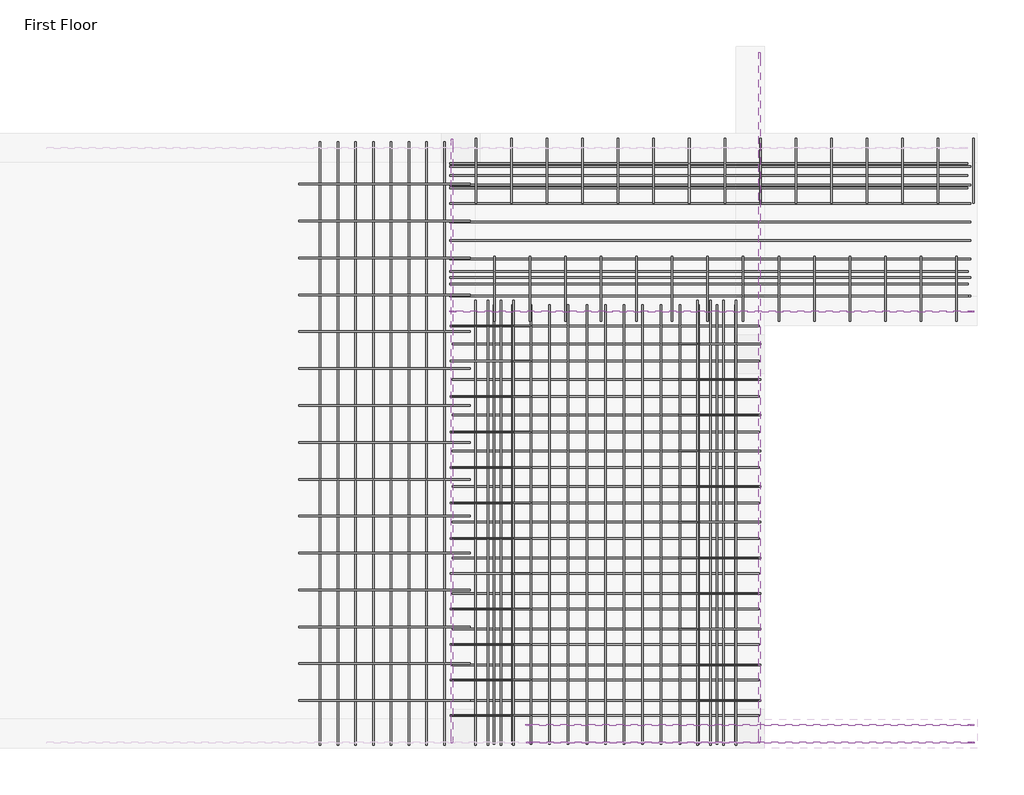
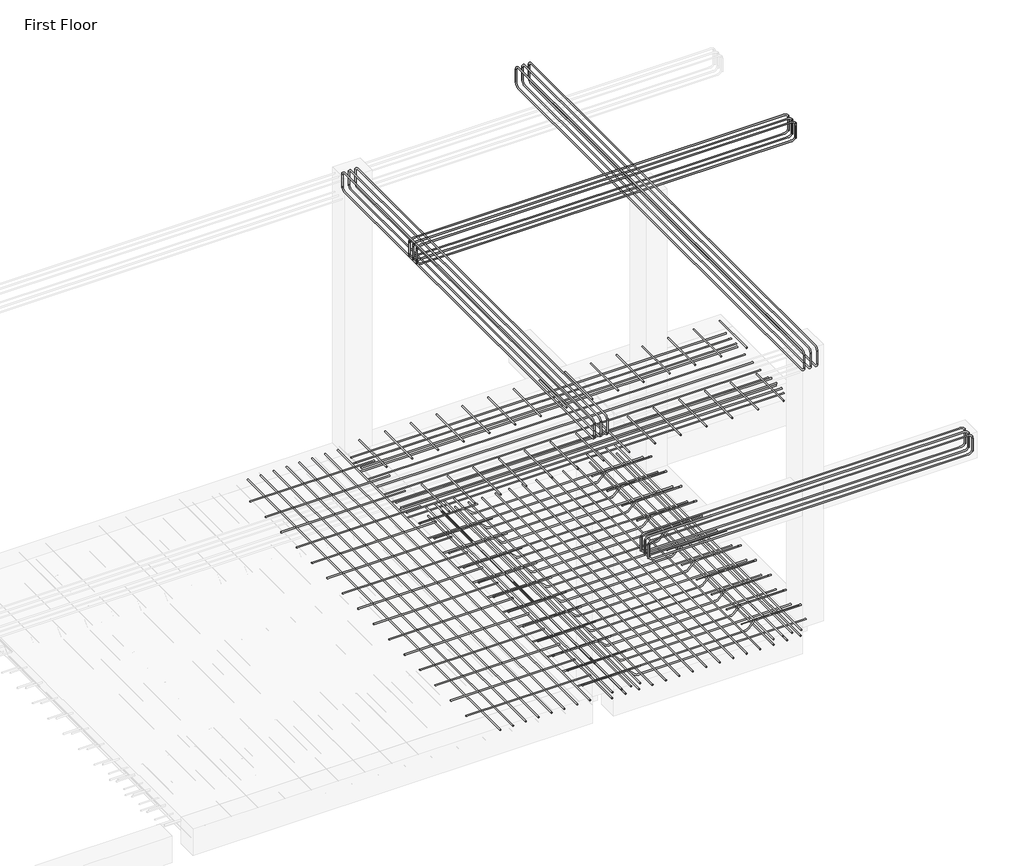
# One storey, part 4 of 4: 22 reinforcing bars.
"""IFC4 building model written with IfcOpenShell, lengths in millimetres."""

from ifc_helpers import new_model, si_unit, point, frame, origin, place, context, project, spatial, polyline, circle_curve, trimmed, segment, composite_curve, source, transform, mapped, element, save
from ifc_brep_helpers import swept_disk

model = new_model("IFC4")

# Units and contexts
model_context = context("Model", 3, world=origin())
ifc_project = project(units=[si_unit("LENGTHUNIT", "METRE", prefix="MILLI")], contexts=[model_context])

# Site, building, storey
site = spatial("IfcSite", under=ifc_project)
building = spatial("IfcBuilding", under=site)
storey = spatial("IfcBuildingStorey", under=building, Name="First Floor", Elevation=3200.4)

# Reinforcing bars
placement = place(None, origin())
reinforcing_bar_shape = source(origin(), model_context, "Body", "SolidModel", [
    swept_disk(composite_curve([segment(polyline([(1700.4887526, 5017.2334631, 6163.6994949), (1700.4887526, 5017.2334631, 6311.6994949)]), True, "CONTINUOUS"), segment(trimmed(circle_curve(frame((1700.4887526, 4971.2334631, 6311.6994949), z_axis=(1.0, 0.0, 0.0), x_axis=(0.0, 46.0, 0.0)), 46.0), [point((1700.4887526, 5017.2334631, 6311.6994949))], [point((1700.4887526, 4971.2334631, 6357.6994949))], True, "CARTESIAN"), True, "CONTINUOUS"), segment(polyline([(1700.4887526, 4971.2334631, 6357.6994949), (1700.4887526, 278.4334631, 6357.6994949)]), True, "CONTINUOUS"), segment(trimmed(circle_curve(frame((1700.4887526, 278.4334631, 6311.6994949), z_axis=(1.0, 0.0, 0.0), x_axis=(0.0, 0.0, 46.0)), 46.0), [point((1700.4887526, 278.4334631, 6357.6994949))], [point((1700.4887526, 232.4334631, 6311.6994949))], True, "CARTESIAN"), True, "CONTINUOUS"), segment(polyline([(1700.4887526, 232.4334631, 6311.6994949), (1700.4887526, 232.4334631, 6163.6994949)]), True, "CONTINUOUS")], self_intersect=False), 6.0),
])
element("IfcReinforcingBar", 1, at=placement, inside=storey, context=model_context, shape_type="MappedRepresentation", body=[
    mapped(reinforcing_bar_shape, transform((0.0, 0.0, 0.0), x_axis=(1.0, 0.0, 0.0), y_axis=(0.0, 1.0, 0.0), z_axis=(0.0, 0.0, 1.0))),
    mapped(reinforcing_bar_shape, transform((71.1994949, 0.0, 0.0), x_axis=(1.0, 0.0, 0.0), y_axis=(0.0, 1.0, 0.0), z_axis=(0.0, 0.0, 1.0))),
    mapped(reinforcing_bar_shape, transform((142.3989899, 0.0, 0.0), x_axis=(1.0, 0.0, 0.0), y_axis=(0.0, 1.0, 0.0), z_axis=(0.0, 0.0, 1.0))),
])
reinforcing_bar_2_shape = source(origin(), model_context, "Body", "SolidModel", [
    swept_disk(composite_curve([segment(polyline([(1700.4887526, 5017.2334631, 6333.1005051), (1700.4887526, 5017.2334631, 6185.1005051)]), True, "CONTINUOUS"), segment(trimmed(circle_curve(frame((1700.4887526, 4971.2334631, 6185.1005051), z_axis=(-1.0, 0.0, 0.0), x_axis=(0.0, 46.0, 0.0)), 46.0), [point((1700.4887526, 5017.2334631, 6185.1005051))], [point((1700.4887526, 4971.2334631, 6139.1005051))], True, "CARTESIAN"), True, "CONTINUOUS"), segment(polyline([(1700.4887526, 4971.2334631, 6139.1005051), (1700.4887526, 278.4334631, 6139.1005051)]), True, "CONTINUOUS"), segment(trimmed(circle_curve(frame((1700.4887526, 278.4334631, 6185.1005051), z_axis=(-1.0, 0.0, 0.0), x_axis=(0.0, 0.0, -46.0)), 46.0), [point((1700.4887526, 278.4334631, 6139.1005051))], [point((1700.4887526, 232.4334631, 6185.1005051))], True, "CARTESIAN"), True, "CONTINUOUS"), segment(polyline([(1700.4887526, 232.4334631, 6185.1005051), (1700.4887526, 232.4334631, 6333.1005051)]), True, "CONTINUOUS")], self_intersect=False), 6.0),
])
element("IfcReinforcingBar", 2, at=placement, inside=storey, context=model_context, shape_type="MappedRepresentation", body=[
    mapped(reinforcing_bar_2_shape, transform((0.0, 0.0, 0.0), x_axis=(1.0, 0.0, 0.0), y_axis=(0.0, 1.0, 0.0), z_axis=(0.0, 0.0, 1.0))),
    mapped(reinforcing_bar_2_shape, transform((71.1994949, 0.0, 0.0), x_axis=(1.0, 0.0, 0.0), y_axis=(0.0, 1.0, 0.0), z_axis=(0.0, 0.0, 1.0))),
    mapped(reinforcing_bar_2_shape, transform((142.3989899, 0.0, 0.0), x_axis=(1.0, 0.0, 0.0), y_axis=(0.0, 1.0, 0.0), z_axis=(0.0, 0.0, 1.0))),
])
reinforcing_bar_3_shape = source(origin(), model_context, "Body", "SolidModel", [
    swept_disk(composite_curve([segment(polyline([(3999.1887526, 5705.3580501, 6163.6994949), (3999.1887526, 5705.3580501, 6311.6994949)]), True, "CONTINUOUS"), segment(trimmed(circle_curve(frame((3999.1887526, 5659.3580501, 6311.6994949), z_axis=(1.0, 0.0, 0.0), x_axis=(0.0, 46.0, 0.0)), 46.0), [point((3999.1887526, 5705.3580501, 6311.6994949))], [point((3999.1887526, 5659.3580501, 6357.6994949))], True, "CARTESIAN"), True, "CONTINUOUS"), segment(polyline([(3999.1887526, 5659.3580501, 6357.6994949), (3999.1887526, 278.4334631, 6357.6994949)]), True, "CONTINUOUS"), segment(trimmed(circle_curve(frame((3999.1887526, 278.4334631, 6311.6994949), z_axis=(1.0, 0.0, 0.0), x_axis=(0.0, 0.0, 46.0)), 46.0), [point((3999.1887526, 278.4334631, 6357.6994949))], [point((3999.1887526, 232.4334631, 6311.6994949))], True, "CARTESIAN"), True, "CONTINUOUS"), segment(polyline([(3999.1887526, 232.4334631, 6311.6994949), (3999.1887526, 232.4334631, 6163.6994949)]), True, "CONTINUOUS")], self_intersect=False), 6.0),
])
element("IfcReinforcingBar", 3, at=placement, inside=storey, context=model_context, shape_type="MappedRepresentation", body=[
    mapped(reinforcing_bar_3_shape, transform((0.0, 0.0, 0.0), x_axis=(1.0, 0.0, 0.0), y_axis=(0.0, 1.0, 0.0), z_axis=(0.0, 0.0, 1.0))),
    mapped(reinforcing_bar_3_shape, transform((71.1994949, 0.0, 0.0), x_axis=(1.0, 0.0, 0.0), y_axis=(0.0, 1.0, 0.0), z_axis=(0.0, 0.0, 1.0))),
    mapped(reinforcing_bar_3_shape, transform((142.3989899, 0.0, 0.0), x_axis=(1.0, 0.0, 0.0), y_axis=(0.0, 1.0, 0.0), z_axis=(0.0, 0.0, 1.0))),
])
reinforcing_bar_4_shape = source(origin(), model_context, "Body", "SolidModel", [
    swept_disk(composite_curve([segment(polyline([(3999.1887526, 5703.3830416, 6318.1005051), (3999.1887526, 5703.3830416, 6170.1005051)]), True, "CONTINUOUS"), segment(trimmed(circle_curve(frame((3999.1887526, 5657.3830416, 6170.1005051), z_axis=(-1.0, 0.0, 0.0), x_axis=(0.0, 46.0, 0.0)), 46.0), [point((3999.1887526, 5703.3830416, 6170.1005051))], [point((3999.1887526, 5657.3830416, 6124.1005051))], True, "CARTESIAN"), True, "CONTINUOUS"), segment(polyline([(3999.1887526, 5657.3830416, 6124.1005051), (3999.1887526, 278.4334631, 6124.1005051)]), True, "CONTINUOUS"), segment(trimmed(circle_curve(frame((3999.1887526, 278.4334631, 6170.1005051), z_axis=(-1.0, 0.0, 0.0), x_axis=(0.0, 0.0, -46.0)), 46.0), [point((3999.1887526, 278.4334631, 6124.1005051))], [point((3999.1887526, 232.4334631, 6170.1005051))], True, "CARTESIAN"), True, "CONTINUOUS"), segment(polyline([(3999.1887526, 232.4334631, 6170.1005051), (3999.1887526, 232.4334631, 6318.1005051)]), True, "CONTINUOUS")], self_intersect=False), 6.0),
])
element("IfcReinforcingBar", 4, at=placement, inside=storey, context=model_context, shape_type="MappedRepresentation", body=[
    mapped(reinforcing_bar_4_shape, transform((0.0, 0.0, 0.0), x_axis=(1.0, 0.0, 0.0), y_axis=(0.0, 1.0, 0.0), z_axis=(0.0, 0.0, 1.0))),
    mapped(reinforcing_bar_4_shape, transform((71.1994949, 0.0, 0.0), x_axis=(1.0, 0.0, 0.0), y_axis=(0.0, 1.0, 0.0), z_axis=(0.0, 0.0, 1.0))),
    mapped(reinforcing_bar_4_shape, transform((142.3989899, 0.0, 0.0), x_axis=(1.0, 0.0, 0.0), y_axis=(0.0, 1.0, 0.0), z_axis=(0.0, 0.0, 1.0))),
])
reinforcing_bar_5_shape = source(origin(), model_context, "Body", "SolidModel", [
    swept_disk(composite_curve([segment(polyline([(5841.2691711, 3584.0814555, 6161.9520076), (5841.2691711, 3584.0814555, 6309.9520076)]), True, "CONTINUOUS"), segment(trimmed(circle_curve(frame((5795.2691711, 3584.0814555, 6309.9520076), z_axis=(0.0, -1.0, 0.0), x_axis=(46.0, 0.0, 0.0)), 46.0), [point((5841.2691711, 3584.0814555, 6309.9520076))], [point((5795.2691711, 3584.0814555, 6355.9520076))], True, "CARTESIAN"), True, "CONTINUOUS"), segment(polyline([(5795.2691711, 3584.0814555, 6355.9520076), (1734.3882476, 3584.0814555, 6355.9520076)]), True, "CONTINUOUS"), segment(trimmed(circle_curve(frame((1734.3882476, 3584.0814555, 6309.9520076), z_axis=(0.0, -1.0, 0.0), x_axis=(0.0, 0.0, 46.0)), 46.0), [point((1734.3882476, 3584.0814555, 6355.9520076))], [point((1688.3882476, 3584.0814555, 6309.9520076))], True, "CARTESIAN"), True, "CONTINUOUS"), segment(polyline([(1688.3882476, 3584.0814555, 6309.9520076), (1688.3882476, 3584.0814555, 6161.9520076)]), True, "CONTINUOUS")], self_intersect=False), 6.0),
])
element("IfcReinforcingBar", 5, at=placement, inside=storey, context=model_context, shape_type="MappedRepresentation", body=[
    mapped(reinforcing_bar_5_shape, transform((0.0, 0.0, 0.0), x_axis=(1.0, 0.0, 0.0), y_axis=(0.0, 1.0, 0.0), z_axis=(0.0, 0.0, 1.0))),
    mapped(reinforcing_bar_5_shape, transform((0.0, 69.4520076, 0.0), x_axis=(1.0, 0.0, 0.0), y_axis=(0.0, 1.0, 0.0), z_axis=(0.0, 0.0, 1.0))),
    mapped(reinforcing_bar_5_shape, transform((0.0, 138.9040151, 0.0), x_axis=(1.0, 0.0, 0.0), y_axis=(0.0, 1.0, 0.0), z_axis=(0.0, 0.0, 1.0))),
])
reinforcing_bar_6_shape = source(origin(), model_context, "Body", "SolidModel", [
    swept_disk(composite_curve([segment(polyline([(5840.2625116, 3584.0814555, 6334.8479924), (5840.2625116, 3584.0814555, 6186.8479924)]), True, "CONTINUOUS"), segment(trimmed(circle_curve(frame((5794.2625116, 3584.0814555, 6186.8479924), z_axis=(0.0, 1.0, 0.0), x_axis=(46.0, 0.0, 0.0)), 46.0), [point((5840.2625116, 3584.0814555, 6186.8479924))], [point((5794.2625116, 3584.0814555, 6140.8479924))], True, "CARTESIAN"), True, "CONTINUOUS"), segment(polyline([(5794.2625116, 3584.0814555, 6140.8479924), (1734.3882476, 3584.0814555, 6140.8479924)]), True, "CONTINUOUS"), segment(trimmed(circle_curve(frame((1734.3882476, 3584.0814555, 6186.8479924), z_axis=(0.0, 1.0, 0.0), x_axis=(0.0, 0.0, -46.0)), 46.0), [point((1734.3882476, 3584.0814555, 6140.8479924))], [point((1688.3882476, 3584.0814555, 6186.8479924))], True, "CARTESIAN"), True, "CONTINUOUS"), segment(polyline([(1688.3882476, 3584.0814555, 6186.8479924), (1688.3882476, 3584.0814555, 6334.8479924)]), True, "CONTINUOUS")], self_intersect=False), 6.0),
])
element("IfcReinforcingBar", 6, at=placement, inside=storey, context=model_context, shape_type="MappedRepresentation", body=[
    mapped(reinforcing_bar_6_shape, transform((0.0, 0.0, 0.0), x_axis=(1.0, 0.0, 0.0), y_axis=(0.0, 1.0, 0.0), z_axis=(0.0, 0.0, 1.0))),
    mapped(reinforcing_bar_6_shape, transform((0.0, 69.4520076, 0.0), x_axis=(1.0, 0.0, 0.0), y_axis=(0.0, 1.0, 0.0), z_axis=(0.0, 0.0, 1.0))),
    mapped(reinforcing_bar_6_shape, transform((0.0, 138.9040151, 0.0), x_axis=(1.0, 0.0, 0.0), y_axis=(0.0, 1.0, 0.0), z_axis=(0.0, 0.0, 1.0))),
])
reinforcing_bar_7_shape = source(origin(), model_context, "Body", "SolidModel", [
    swept_disk(composite_curve([segment(polyline([(5841.2691711, 229.5339681, 4563.4994949), (5841.2691711, 229.5339681, 4711.4994949)]), True, "CONTINUOUS"), segment(trimmed(circle_curve(frame((5795.2691711, 229.5339681, 4711.4994949), z_axis=(0.0, -1.0, 0.0), x_axis=(46.0, 0.0, 0.0)), 46.0), [point((5841.2691711, 229.5339681, 4711.4994949))], [point((5795.2691711, 229.5339681, 4757.4994949))], True, "CARTESIAN"), True, "CONTINUOUS"), segment(polyline([(5795.2691711, 229.5339681, 4757.4994949), (2337.5636354, 229.5339681, 4757.4994949)]), True, "CONTINUOUS"), segment(trimmed(circle_curve(frame((2337.5636354, 229.5339681, 4711.4994949), z_axis=(0.0, -1.0, 0.0), x_axis=(0.0, 0.0, 46.0)), 46.0), [point((2337.5636354, 229.5339681, 4757.4994949))], [point((2291.5636354, 229.5339681, 4711.4994949))], True, "CARTESIAN"), True, "CONTINUOUS"), segment(polyline([(2291.5636354, 229.5339681, 4711.4994949), (2291.5636354, 229.5339681, 4563.4994949)]), True, "CONTINUOUS")], self_intersect=False), 6.0),
])
element("IfcReinforcingBar", 7, at=placement, inside=storey, context=model_context, shape_type="MappedRepresentation", body=[
    mapped(reinforcing_bar_7_shape, transform((0.0, 0.0, 0.0), x_axis=(1.0, 0.0, 0.0), y_axis=(0.0, 1.0, 0.0), z_axis=(0.0, 0.0, 1.0))),
    mapped(reinforcing_bar_7_shape, transform((0.0, 71.1994949, 0.0), x_axis=(1.0, 0.0, 0.0), y_axis=(0.0, 1.0, 0.0), z_axis=(0.0, 0.0, 1.0))),
    mapped(reinforcing_bar_7_shape, transform((0.0, 142.3989899, 0.0), x_axis=(1.0, 0.0, 0.0), y_axis=(0.0, 1.0, 0.0), z_axis=(0.0, 0.0, 1.0))),
])
reinforcing_bar_8_shape = source(origin(), model_context, "Body", "SolidModel", [
    swept_disk(composite_curve([segment(polyline([(5840.2625116, 229.5339681, 4732.9005051), (5840.2625116, 229.5339681, 4584.9005051)]), True, "CONTINUOUS"), segment(trimmed(circle_curve(frame((5794.2625116, 229.5339681, 4584.9005051), z_axis=(0.0, 1.0, 0.0), x_axis=(46.0, 0.0, 0.0)), 46.0), [point((5840.2625116, 229.5339681, 4584.9005051))], [point((5794.2625116, 229.5339681, 4538.9005051))], True, "CARTESIAN"), True, "CONTINUOUS"), segment(polyline([(5794.2625116, 229.5339681, 4538.9005051), (2341.190873, 229.5339681, 4538.9005051)]), True, "CONTINUOUS"), segment(trimmed(circle_curve(frame((2341.190873, 229.5339681, 4584.9005051), z_axis=(0.0, 1.0, 0.0), x_axis=(0.0, 0.0, -46.0)), 46.0), [point((2341.190873, 229.5339681, 4538.9005051))], [point((2295.190873, 229.5339681, 4584.9005051))], True, "CARTESIAN"), True, "CONTINUOUS"), segment(polyline([(2295.190873, 229.5339681, 4584.9005051), (2295.190873, 229.5339681, 4732.9005051)]), True, "CONTINUOUS")], self_intersect=False), 6.0),
])
element("IfcReinforcingBar", 8, at=placement, inside=storey, context=model_context, shape_type="MappedRepresentation", body=[
    mapped(reinforcing_bar_8_shape, transform((0.0, 0.0, 0.0), x_axis=(1.0, 0.0, 0.0), y_axis=(0.0, 1.0, 0.0), z_axis=(0.0, 0.0, 1.0))),
    mapped(reinforcing_bar_8_shape, transform((0.0, 71.1994949, 0.0), x_axis=(1.0, 0.0, 0.0), y_axis=(0.0, 1.0, 0.0), z_axis=(0.0, 0.0, 1.0))),
    mapped(reinforcing_bar_8_shape, transform((0.0, 142.3989899, 0.0), x_axis=(1.0, 0.0, 0.0), y_axis=(0.0, 1.0, 0.0), z_axis=(0.0, 0.0, 1.0))),
])
reinforcing_bar_9_shape = source(origin(), model_context, "Body", "SolidModel", [
    swept_disk(composite_curve([segment(polyline([(1688.7874305, 3539.2334631, 3169.4), (2168.5956769, 3539.2334631, 3169.4)]), True, "CONTINUOUS"), segment(trimmed(circle_curve(frame((2168.5956769, 3539.2334631, 3123.4), z_axis=(0.0, 1.0, 0.0), x_axis=(0.0, 0.0, 46.0)), 46.0), [point((2168.5956769, 3539.2334631, 3169.4))], [point((2201.1225888, 3539.2334631, 3155.9269119))], True, "CARTESIAN"), True, "CONTINUOUS"), segment(polyline([(2201.1225888, 3539.2334631, 3155.9269119), (2264.5764127, 3539.2334631, 3092.4730881)]), True, "CONTINUOUS"), segment(trimmed(circle_curve(frame((2297.1033246, 3539.2334631, 3125.0), z_axis=(0.0, -1.0, 0.0), x_axis=(-32.52691189999996, 0.0, -32.52691189999996)), 46.0), [point((2264.5764127, 3539.2334631, 3092.4730881))], [point((2297.1033246, 3539.2334631, 3079.0))], True, "CARTESIAN"), True, "CONTINUOUS"), segment(polyline([(2297.1033246, 3539.2334631, 3079.0), (4139.8402551, 3539.2334631, 3079.0)]), True, "CONTINUOUS")], self_intersect=False), 6.0),
])
element("IfcReinforcingBar", 9, at=placement, inside=storey, context=model_context, shape_type="MappedRepresentation", body=[
    mapped(reinforcing_bar_9_shape, transform((0.0, 0.0, 0.0), x_axis=(1.0, 0.0, 0.0), y_axis=(0.0, 1.0, 0.0), z_axis=(0.0, 0.0, 1.0))),
    mapped(reinforcing_bar_9_shape, transform((0.0, -281.0909091, 0.0), x_axis=(1.0, 0.0, 0.0), y_axis=(0.0, 1.0, 0.0), z_axis=(0.0, 0.0, 1.0))),
    mapped(reinforcing_bar_9_shape, transform((0.0, -562.1818182, 0.0), x_axis=(1.0, 0.0, 0.0), y_axis=(0.0, 1.0, 0.0), z_axis=(0.0, 0.0, 1.0))),
    mapped(reinforcing_bar_9_shape, transform((0.0, -843.2727273, 0.0), x_axis=(1.0, 0.0, 0.0), y_axis=(0.0, 1.0, 0.0), z_axis=(0.0, 0.0, 1.0))),
    mapped(reinforcing_bar_9_shape, transform((0.0, -1124.3636364, 0.0), x_axis=(1.0, 0.0, 0.0), y_axis=(0.0, 1.0, 0.0), z_axis=(0.0, 0.0, 1.0))),
    mapped(reinforcing_bar_9_shape, transform((0.0, -1405.4545455, 0.0), x_axis=(1.0, 0.0, 0.0), y_axis=(0.0, 1.0, 0.0), z_axis=(0.0, 0.0, 1.0))),
    mapped(reinforcing_bar_9_shape, transform((0.0, -1686.5454545, 0.0), x_axis=(1.0, 0.0, 0.0), y_axis=(0.0, 1.0, 0.0), z_axis=(0.0, 0.0, 1.0))),
    mapped(reinforcing_bar_9_shape, transform((0.0, -1967.6363636, 0.0), x_axis=(1.0, 0.0, 0.0), y_axis=(0.0, 1.0, 0.0), z_axis=(0.0, 0.0, 1.0))),
    mapped(reinforcing_bar_9_shape, transform((0.0, -2248.7272727, 0.0), x_axis=(1.0, 0.0, 0.0), y_axis=(0.0, 1.0, 0.0), z_axis=(0.0, 0.0, 1.0))),
    mapped(reinforcing_bar_9_shape, transform((0.0, -2529.8181818, 0.0), x_axis=(1.0, 0.0, 0.0), y_axis=(0.0, 1.0, 0.0), z_axis=(0.0, 0.0, 1.0))),
    mapped(reinforcing_bar_9_shape, transform((0.0, -2810.9090909, 0.0), x_axis=(1.0, 0.0, 0.0), y_axis=(0.0, 1.0, 0.0), z_axis=(0.0, 0.0, 1.0))),
    mapped(reinforcing_bar_9_shape, transform((0.0, -3092.0, 0.0), x_axis=(1.0, 0.0, 0.0), y_axis=(0.0, 1.0, 0.0), z_axis=(0.0, 0.0, 1.0))),
])
reinforcing_bar_10_shape = source(origin(), model_context, "Body", "SolidModel", [
    swept_disk(composite_curve([segment(polyline([(4153.2890646, 564.2307141, 3169.4), (3672.2951557, 564.2307141, 3169.4)]), True, "CONTINUOUS"), segment(trimmed(circle_curve(frame((3672.2951557, 564.2307141, 3123.4), z_axis=(0.0, -1.0, 0.0), x_axis=(0.0, 0.0, 46.0)), 46.0), [point((3672.2951557, 564.2307141, 3169.4))], [point((3639.7682438, 564.2307141, 3155.9269119))], True, "CARTESIAN"), True, "CONTINUOUS"), segment(polyline([(3639.7682438, 564.2307141, 3155.9269119), (3576.3144199, 564.2307141, 3092.4730881)]), True, "CONTINUOUS"), segment(trimmed(circle_curve(frame((3543.787508, 564.2307141, 3125.0), z_axis=(0.0, 1.0000000000000002, 0.0), x_axis=(32.52691189999996, 0.0, -32.52691189999996)), 46.0), [point((3576.3144199, 564.2307141, 3092.4730881))], [point((3543.787508, 564.2307141, 3079.0))], True, "CARTESIAN"), True, "CONTINUOUS"), segment(polyline([(3543.787508, 564.2307141, 3079.0), (1702.23624, 564.2307141, 3079.0)]), True, "CONTINUOUS")], self_intersect=False), 6.0),
])
element("IfcReinforcingBar", 10, at=placement, inside=storey, context=model_context, shape_type="MappedRepresentation", body=[
    mapped(reinforcing_bar_10_shape, transform((0.0, 0.0, 0.0), x_axis=(1.0, 0.0, 0.0), y_axis=(0.0, 1.0, 0.0), z_axis=(0.0, 0.0, 1.0))),
    mapped(reinforcing_bar_10_shape, transform((0.0, 283.1945647, 0.0), x_axis=(1.0, 0.0, 0.0), y_axis=(0.0, 1.0, 0.0), z_axis=(0.0, 0.0, 1.0))),
    mapped(reinforcing_bar_10_shape, transform((0.0, 566.3891295, 0.0), x_axis=(1.0, 0.0, 0.0), y_axis=(0.0, 1.0, 0.0), z_axis=(0.0, 0.0, 1.0))),
    mapped(reinforcing_bar_10_shape, transform((0.0, 849.5836942, 0.0), x_axis=(1.0, 0.0, 0.0), y_axis=(0.0, 1.0, 0.0), z_axis=(0.0, 0.0, 1.0))),
    mapped(reinforcing_bar_10_shape, transform((0.0, 1132.778259, 0.0), x_axis=(1.0, 0.0, 0.0), y_axis=(0.0, 1.0, 0.0), z_axis=(0.0, 0.0, 1.0))),
    mapped(reinforcing_bar_10_shape, transform((0.0, 1415.9728237, 0.0), x_axis=(1.0, 0.0, 0.0), y_axis=(0.0, 1.0, 0.0), z_axis=(0.0, 0.0, 1.0))),
    mapped(reinforcing_bar_10_shape, transform((0.0, 1699.1673885, 0.0), x_axis=(1.0, 0.0, 0.0), y_axis=(0.0, 1.0, 0.0), z_axis=(0.0, 0.0, 1.0))),
    mapped(reinforcing_bar_10_shape, transform((0.0, 1982.3619532, 0.0), x_axis=(1.0, 0.0, 0.0), y_axis=(0.0, 1.0, 0.0), z_axis=(0.0, 0.0, 1.0))),
    mapped(reinforcing_bar_10_shape, transform((0.0, 2265.556518, 0.0), x_axis=(1.0, 0.0, 0.0), y_axis=(0.0, 1.0, 0.0), z_axis=(0.0, 0.0, 1.0))),
    mapped(reinforcing_bar_10_shape, transform((0.0, 2548.7510827, 0.0), x_axis=(1.0, 0.0, 0.0), y_axis=(0.0, 1.0, 0.0), z_axis=(0.0, 0.0, 1.0))),
    mapped(reinforcing_bar_10_shape, transform((0.0, 2831.9456475, 0.0), x_axis=(1.0, 0.0, 0.0), y_axis=(0.0, 1.0, 0.0), z_axis=(0.0, 0.0, 1.0))),
])
reinforcing_bar_11_shape = source(origin(), model_context, "Body", "SolidModel", [
    swept_disk(composite_curve([segment(polyline([(3650.7560505, 3742.8334631, 3159.1006995), (3650.7560505, 211.4334631, 3159.1006995)]), True, "CONTINUOUS")], self_intersect=False), 6.0),
])
element("IfcReinforcingBar", 11, at=placement, inside=storey, context=model_context, shape_type="MappedRepresentation", body=[
    mapped(reinforcing_bar_11_shape, transform((0.0, 0.0, 0.0), x_axis=(1.0, 0.0, 0.0), y_axis=(0.0, 1.0, 0.0), z_axis=(0.0, 0.0, 1.0))),
    mapped(reinforcing_bar_11_shape, transform((101.777399, 0.0, 0.0), x_axis=(1.0, 0.0, 0.0), y_axis=(0.0, 1.0, 0.0), z_axis=(0.0, 0.0, 1.0))),
    mapped(reinforcing_bar_11_shape, transform((203.554798, 0.0, 0.0), x_axis=(1.0, 0.0, 0.0), y_axis=(0.0, 1.0, 0.0), z_axis=(0.0, 0.0, 1.0))),
    mapped(reinforcing_bar_11_shape, transform((305.3321971, 0.0, 0.0), x_axis=(1.0, 0.0, 0.0), y_axis=(0.0, 1.0, 0.0), z_axis=(0.0, 0.0, 1.0))),
])
reinforcing_bar_12_shape = source(origin(), model_context, "Body", "SolidModel", [
    swept_disk(composite_curve([segment(polyline([(1697.8477074, 3539.2334631, 3171.4), (2325.3671503, 3539.2334631, 3171.4)]), True, "CONTINUOUS")], self_intersect=False), 4.0),
])
element("IfcReinforcingBar", 12, at=placement, inside=storey, context=model_context, shape_type="MappedRepresentation", body=[
    mapped(reinforcing_bar_12_shape, transform((0.0, 0.0, 0.0), x_axis=(1.0, 0.0, 0.0), y_axis=(0.0, 1.0, 0.0), z_axis=(0.0, 0.0, 1.0))),
    mapped(reinforcing_bar_12_shape, transform((0.0, -281.0909091, 0.0), x_axis=(1.0, 0.0, 0.0), y_axis=(0.0, 1.0, 0.0), z_axis=(0.0, 0.0, 1.0))),
    mapped(reinforcing_bar_12_shape, transform((0.0, -562.1818182, 0.0), x_axis=(1.0, 0.0, 0.0), y_axis=(0.0, 1.0, 0.0), z_axis=(0.0, 0.0, 1.0))),
    mapped(reinforcing_bar_12_shape, transform((0.0, -843.2727273, 0.0), x_axis=(1.0, 0.0, 0.0), y_axis=(0.0, 1.0, 0.0), z_axis=(0.0, 0.0, 1.0))),
    mapped(reinforcing_bar_12_shape, transform((0.0, -1124.3636364, 0.0), x_axis=(1.0, 0.0, 0.0), y_axis=(0.0, 1.0, 0.0), z_axis=(0.0, 0.0, 1.0))),
    mapped(reinforcing_bar_12_shape, transform((0.0, -1405.4545455, 0.0), x_axis=(1.0, 0.0, 0.0), y_axis=(0.0, 1.0, 0.0), z_axis=(0.0, 0.0, 1.0))),
    mapped(reinforcing_bar_12_shape, transform((0.0, -1686.5454545, 0.0), x_axis=(1.0, 0.0, 0.0), y_axis=(0.0, 1.0, 0.0), z_axis=(0.0, 0.0, 1.0))),
    mapped(reinforcing_bar_12_shape, transform((0.0, -1967.6363636, 0.0), x_axis=(1.0, 0.0, 0.0), y_axis=(0.0, 1.0, 0.0), z_axis=(0.0, 0.0, 1.0))),
    mapped(reinforcing_bar_12_shape, transform((0.0, -2248.7272727, 0.0), x_axis=(1.0, 0.0, 0.0), y_axis=(0.0, 1.0, 0.0), z_axis=(0.0, 0.0, 1.0))),
    mapped(reinforcing_bar_12_shape, transform((0.0, -2529.8181818, 0.0), x_axis=(1.0, 0.0, 0.0), y_axis=(0.0, 1.0, 0.0), z_axis=(0.0, 0.0, 1.0))),
    mapped(reinforcing_bar_12_shape, transform((0.0, -2810.9090909, 0.0), x_axis=(1.0, 0.0, 0.0), y_axis=(0.0, 1.0, 0.0), z_axis=(0.0, 0.0, 1.0))),
    mapped(reinforcing_bar_12_shape, transform((0.0, -3092.0, 0.0), x_axis=(1.0, 0.0, 0.0), y_axis=(0.0, 1.0, 0.0), z_axis=(0.0, 0.0, 1.0))),
])
reinforcing_bar_13_shape = source(origin(), model_context, "Body", "SolidModel", [
    swept_disk(composite_curve([segment(polyline([(4130.5876361, 3396.1763616, 3171.4), (3500.3340616, 3396.1763616, 3171.4)]), True, "CONTINUOUS")], self_intersect=False), 4.0),
])
element("IfcReinforcingBar", 13, at=placement, inside=storey, context=model_context, shape_type="MappedRepresentation", body=[
    mapped(reinforcing_bar_13_shape, transform((0.0, 0.0, 0.0), x_axis=(1.0, 0.0, 0.0), y_axis=(0.0, 1.0, 0.0), z_axis=(0.0, 0.0, 1.0))),
    mapped(reinforcing_bar_13_shape, transform((0.0, -283.1945647, 0.0), x_axis=(1.0, 0.0, 0.0), y_axis=(0.0, 1.0, 0.0), z_axis=(0.0, 0.0, 1.0))),
    mapped(reinforcing_bar_13_shape, transform((0.0, -566.3891295, 0.0), x_axis=(1.0, 0.0, 0.0), y_axis=(0.0, 1.0, 0.0), z_axis=(0.0, 0.0, 1.0))),
    mapped(reinforcing_bar_13_shape, transform((0.0, -849.5836942, 0.0), x_axis=(1.0, 0.0, 0.0), y_axis=(0.0, 1.0, 0.0), z_axis=(0.0, 0.0, 1.0))),
    mapped(reinforcing_bar_13_shape, transform((0.0, -1132.778259, 0.0), x_axis=(1.0, 0.0, 0.0), y_axis=(0.0, 1.0, 0.0), z_axis=(0.0, 0.0, 1.0))),
    mapped(reinforcing_bar_13_shape, transform((0.0, -1415.9728237, 0.0), x_axis=(1.0, 0.0, 0.0), y_axis=(0.0, 1.0, 0.0), z_axis=(0.0, 0.0, 1.0))),
    mapped(reinforcing_bar_13_shape, transform((0.0, -1699.1673885, 0.0), x_axis=(1.0, 0.0, 0.0), y_axis=(0.0, 1.0, 0.0), z_axis=(0.0, 0.0, 1.0))),
    mapped(reinforcing_bar_13_shape, transform((0.0, -1982.3619532, 0.0), x_axis=(1.0, 0.0, 0.0), y_axis=(0.0, 1.0, 0.0), z_axis=(0.0, 0.0, 1.0))),
    mapped(reinforcing_bar_13_shape, transform((0.0, -2265.556518, 0.0), x_axis=(1.0, 0.0, 0.0), y_axis=(0.0, 1.0, 0.0), z_axis=(0.0, 0.0, 1.0))),
    mapped(reinforcing_bar_13_shape, transform((0.0, -2548.7510827, 0.0), x_axis=(1.0, 0.0, 0.0), y_axis=(0.0, 1.0, 0.0), z_axis=(0.0, 0.0, 1.0))),
    mapped(reinforcing_bar_13_shape, transform((0.0, -2831.9456475, 0.0), x_axis=(1.0, 0.0, 0.0), y_axis=(0.0, 1.0, 0.0), z_axis=(0.0, 0.0, 1.0))),
])
reinforcing_bar_14_shape = source(origin(), model_context, "Body", "SolidModel", [
    swept_disk(composite_curve([segment(polyline([(3952.0882476, 218.9117605, 3087.5387401), (3952.0882476, 3706.6679133, 3087.5387401)]), True, "CONTINUOUS")], self_intersect=False), 6.0),
])
element("IfcReinforcingBar", 14, at=placement, inside=storey, context=model_context, shape_type="MappedRepresentation", body=[
    mapped(reinforcing_bar_14_shape, transform((0.0, 0.0, 0.0), x_axis=(1.0, 0.0, 0.0), y_axis=(0.0, 1.0, 0.0), z_axis=(0.0, 0.0, 1.0))),
    mapped(reinforcing_bar_14_shape, transform((-147.5785714, 0.0, 0.0), x_axis=(1.0, 0.0, 0.0), y_axis=(0.0, 1.0, 0.0), z_axis=(0.0, 0.0, 1.0))),
    mapped(reinforcing_bar_14_shape, transform((-295.1571429, 0.0, 0.0), x_axis=(1.0, 0.0, 0.0), y_axis=(0.0, 1.0, 0.0), z_axis=(0.0, 0.0, 1.0))),
    mapped(reinforcing_bar_14_shape, transform((-442.7357143, 0.0, 0.0), x_axis=(1.0, 0.0, 0.0), y_axis=(0.0, 1.0, 0.0), z_axis=(0.0, 0.0, 1.0))),
    mapped(reinforcing_bar_14_shape, transform((-590.3142857, 0.0, 0.0), x_axis=(1.0, 0.0, 0.0), y_axis=(0.0, 1.0, 0.0), z_axis=(0.0, 0.0, 1.0))),
    mapped(reinforcing_bar_14_shape, transform((-737.8928571, 0.0, 0.0), x_axis=(1.0, 0.0, 0.0), y_axis=(0.0, 1.0, 0.0), z_axis=(0.0, 0.0, 1.0))),
    mapped(reinforcing_bar_14_shape, transform((-885.4714286, 0.0, 0.0), x_axis=(1.0, 0.0, 0.0), y_axis=(0.0, 1.0, 0.0), z_axis=(0.0, 0.0, 1.0))),
    mapped(reinforcing_bar_14_shape, transform((-1033.05, 0.0, 0.0), x_axis=(1.0, 0.0, 0.0), y_axis=(0.0, 1.0, 0.0), z_axis=(0.0, 0.0, 1.0))),
    mapped(reinforcing_bar_14_shape, transform((-1180.6285714, 0.0, 0.0), x_axis=(1.0, 0.0, 0.0), y_axis=(0.0, 1.0, 0.0), z_axis=(0.0, 0.0, 1.0))),
    mapped(reinforcing_bar_14_shape, transform((-1328.2071429, 0.0, 0.0), x_axis=(1.0, 0.0, 0.0), y_axis=(0.0, 1.0, 0.0), z_axis=(0.0, 0.0, 1.0))),
    mapped(reinforcing_bar_14_shape, transform((-1475.7857143, 0.0, 0.0), x_axis=(1.0, 0.0, 0.0), y_axis=(0.0, 1.0, 0.0), z_axis=(0.0, 0.0, 1.0))),
    mapped(reinforcing_bar_14_shape, transform((-1623.3642857, 0.0, 0.0), x_axis=(1.0, 0.0, 0.0), y_axis=(0.0, 1.0, 0.0), z_axis=(0.0, 0.0, 1.0))),
    mapped(reinforcing_bar_14_shape, transform((-1770.9428571, 0.0, 0.0), x_axis=(1.0, 0.0, 0.0), y_axis=(0.0, 1.0, 0.0), z_axis=(0.0, 0.0, 1.0))),
    mapped(reinforcing_bar_14_shape, transform((-1918.5214286, 0.0, 0.0), x_axis=(1.0, 0.0, 0.0), y_axis=(0.0, 1.0, 0.0), z_axis=(0.0, 0.0, 1.0))),
    mapped(reinforcing_bar_14_shape, transform((-2066.1, 0.0, 0.0), x_axis=(1.0, 0.0, 0.0), y_axis=(0.0, 1.0, 0.0), z_axis=(0.0, 0.0, 1.0))),
])
reinforcing_bar_15_shape = source(origin(), model_context, "Body", "SolidModel", [
    swept_disk(composite_curve([segment(polyline([(2190.1347821, 3742.8334631, 3159.1006995), (2190.1347821, 211.4334631, 3159.1006995)]), True, "CONTINUOUS")], self_intersect=False), 6.0),
])
element("IfcReinforcingBar", 15, at=placement, inside=storey, context=model_context, shape_type="MappedRepresentation", body=[
    mapped(reinforcing_bar_15_shape, transform((0.0, 0.0, 0.0), x_axis=(1.0, 0.0, 0.0), y_axis=(0.0, 1.0, 0.0), z_axis=(0.0, 0.0, 1.0))),
    mapped(reinforcing_bar_15_shape, transform((-101.3821782, 0.0, 0.0), x_axis=(1.0, 0.0, 0.0), y_axis=(0.0, 1.0, 0.0), z_axis=(0.0, 0.0, 1.0))),
    mapped(reinforcing_bar_15_shape, transform((-202.7643564, 0.0, 0.0), x_axis=(1.0, 0.0, 0.0), y_axis=(0.0, 1.0, 0.0), z_axis=(0.0, 0.0, 1.0))),
    mapped(reinforcing_bar_15_shape, transform((-304.1465345, 0.0, 0.0), x_axis=(1.0, 0.0, 0.0), y_axis=(0.0, 1.0, 0.0), z_axis=(0.0, 0.0, 1.0))),
])
reinforcing_bar_16_shape = source(origin(), model_context, "Body", "SolidModel", [
    swept_disk(composite_curve([segment(polyline([(654.4332967, 4999.0798317, 3154.4697281), (654.4332967, 211.4334631, 3154.4697281)]), True, "CONTINUOUS")], self_intersect=False), 6.0),
])
element("IfcReinforcingBar", 16, at=placement, inside=storey, context=model_context, shape_type="MappedRepresentation", body=[
    mapped(reinforcing_bar_16_shape, transform((0.0, 0.0, 0.0), x_axis=(1.0, 0.0, 0.0), y_axis=(0.0, 1.0, 0.0), z_axis=(0.0, 0.0, 1.0))),
    mapped(reinforcing_bar_16_shape, transform((140.8412233, 0.0, 0.0), x_axis=(1.0, 0.0, 0.0), y_axis=(0.0, 1.0, 0.0), z_axis=(0.0, 0.0, 1.0))),
    mapped(reinforcing_bar_16_shape, transform((281.6824466, 0.0, 0.0), x_axis=(1.0, 0.0, 0.0), y_axis=(0.0, 1.0, 0.0), z_axis=(0.0, 0.0, 1.0))),
    mapped(reinforcing_bar_16_shape, transform((422.5236699, 0.0, 0.0), x_axis=(1.0, 0.0, 0.0), y_axis=(0.0, 1.0, 0.0), z_axis=(0.0, 0.0, 1.0))),
    mapped(reinforcing_bar_16_shape, transform((563.3648932, 0.0, 0.0), x_axis=(1.0, 0.0, 0.0), y_axis=(0.0, 1.0, 0.0), z_axis=(0.0, 0.0, 1.0))),
    mapped(reinforcing_bar_16_shape, transform((704.2061164, 0.0, 0.0), x_axis=(1.0, 0.0, 0.0), y_axis=(0.0, 1.0, 0.0), z_axis=(0.0, 0.0, 1.0))),
    mapped(reinforcing_bar_16_shape, transform((845.0473397, 0.0, 0.0), x_axis=(1.0, 0.0, 0.0), y_axis=(0.0, 1.0, 0.0), z_axis=(0.0, 0.0, 1.0))),
    mapped(reinforcing_bar_16_shape, transform((985.888563, 0.0, 0.0), x_axis=(1.0, 0.0, 0.0), y_axis=(0.0, 1.0, 0.0), z_axis=(0.0, 0.0, 1.0))),
])
reinforcing_bar_17_shape = source(origin(), model_context, "Body", "SolidModel", [
    swept_disk(composite_curve([segment(polyline([(1844.9074635, 564.2307141, 3163.8017937), (483.2910842, 564.2307141, 3163.8017937)]), True, "CONTINUOUS")], self_intersect=False), 6.0),
])
element("IfcReinforcingBar", 17, at=placement, inside=storey, context=model_context, shape_type="MappedRepresentation", body=[
    mapped(reinforcing_bar_17_shape, transform((0.0, 0.0, 0.0), x_axis=(1.0, 0.0, 0.0), y_axis=(0.0, 1.0, 0.0), z_axis=(0.0, 0.0, 1.0))),
    mapped(reinforcing_bar_17_shape, transform((0.0, 292.7783831, 0.0), x_axis=(1.0, 0.0, 0.0), y_axis=(0.0, 1.0, 0.0), z_axis=(0.0, 0.0, 1.0))),
    mapped(reinforcing_bar_17_shape, transform((0.0, 585.5567661, 0.0), x_axis=(1.0, 0.0, 0.0), y_axis=(0.0, 1.0, 0.0), z_axis=(0.0, 0.0, 1.0))),
    mapped(reinforcing_bar_17_shape, transform((0.0, 878.3351492, 0.0), x_axis=(1.0, 0.0, 0.0), y_axis=(0.0, 1.0, 0.0), z_axis=(0.0, 0.0, 1.0))),
    mapped(reinforcing_bar_17_shape, transform((0.0, 1171.1135323, 0.0), x_axis=(1.0, 0.0, 0.0), y_axis=(0.0, 1.0, 0.0), z_axis=(0.0, 0.0, 1.0))),
    mapped(reinforcing_bar_17_shape, transform((0.0, 1463.8919154, 0.0), x_axis=(1.0, 0.0, 0.0), y_axis=(0.0, 1.0, 0.0), z_axis=(0.0, 0.0, 1.0))),
    mapped(reinforcing_bar_17_shape, transform((0.0, 1756.6702984, 0.0), x_axis=(1.0, 0.0, 0.0), y_axis=(0.0, 1.0, 0.0), z_axis=(0.0, 0.0, 1.0))),
    mapped(reinforcing_bar_17_shape, transform((0.0, 2049.4486815, 0.0), x_axis=(1.0, 0.0, 0.0), y_axis=(0.0, 1.0, 0.0), z_axis=(0.0, 0.0, 1.0))),
    mapped(reinforcing_bar_17_shape, transform((0.0, 2342.2270646, 0.0), x_axis=(1.0, 0.0, 0.0), y_axis=(0.0, 1.0, 0.0), z_axis=(0.0, 0.0, 1.0))),
    mapped(reinforcing_bar_17_shape, transform((0.0, 2635.0054477, 0.0), x_axis=(1.0, 0.0, 0.0), y_axis=(0.0, 1.0, 0.0), z_axis=(0.0, 0.0, 1.0))),
    mapped(reinforcing_bar_17_shape, transform((0.0, 2927.7838307, 0.0), x_axis=(1.0, 0.0, 0.0), y_axis=(0.0, 1.0, 0.0), z_axis=(0.0, 0.0, 1.0))),
    mapped(reinforcing_bar_17_shape, transform((0.0, 3220.5622138, 0.0), x_axis=(1.0, 0.0, 0.0), y_axis=(0.0, 1.0, 0.0), z_axis=(0.0, 0.0, 1.0))),
    mapped(reinforcing_bar_17_shape, transform((0.0, 3513.3405969, 0.0), x_axis=(1.0, 0.0, 0.0), y_axis=(0.0, 1.0, 0.0), z_axis=(0.0, 0.0, 1.0))),
    mapped(reinforcing_bar_17_shape, transform((0.0, 3806.11898, 0.0), x_axis=(1.0, 0.0, 0.0), y_axis=(0.0, 1.0, 0.0), z_axis=(0.0, 0.0, 1.0))),
    mapped(reinforcing_bar_17_shape, transform((0.0, 4098.897363, 0.0), x_axis=(1.0, 0.0, 0.0), y_axis=(0.0, 1.0, 0.0), z_axis=(0.0, 0.0, 1.0))),
])
reinforcing_bar_18_shape = source(origin(), model_context, "Body", "SolidModel", [
    swept_disk(composite_curve([segment(polyline([(5796.3354159, 4634.2611065, 3154.3212824), (1682.3882476, 4634.2611065, 3154.3212824)]), True, "CONTINUOUS")], self_intersect=False), 6.0),
])
element("IfcReinforcingBar", 18, at=placement, inside=storey, context=model_context, shape_type="MappedRepresentation", body=[
    mapped(reinforcing_bar_18_shape, transform((0.0, 0.0, 0.0), x_axis=(1.0, 0.0, 0.0), y_axis=(0.0, 1.0, 0.0), z_axis=(0.0, 0.0, 1.0))),
    mapped(reinforcing_bar_18_shape, transform((0.0, 96.3869435, 0.0), x_axis=(1.0, 0.0, 0.0), y_axis=(0.0, 1.0, 0.0), z_axis=(0.0, 0.0, 1.0))),
    mapped(reinforcing_bar_18_shape, transform((0.0, 192.773887, 0.0), x_axis=(1.0, 0.0, 0.0), y_axis=(0.0, 1.0, 0.0), z_axis=(0.0, 0.0, 1.0))),
])
reinforcing_bar_19_shape = source(origin(), model_context, "Body", "SolidModel", [
    swept_disk(composite_curve([segment(polyline([(5798.6824692, 3968.2058196, 3154.3212824), (1682.3882476, 3968.2058196, 3154.3212824)]), True, "CONTINUOUS")], self_intersect=False), 6.0),
])
element("IfcReinforcingBar", 19, at=placement, inside=storey, context=model_context, shape_type="MappedRepresentation", body=[
    mapped(reinforcing_bar_19_shape, transform((0.0, 0.0, 0.0), x_axis=(1.0, 0.0, 0.0), y_axis=(0.0, 1.0, 0.0), z_axis=(0.0, 0.0, 1.0))),
    mapped(reinforcing_bar_19_shape, transform((0.0, -96.3869435, 0.0), x_axis=(1.0, 0.0, 0.0), y_axis=(0.0, 1.0, 0.0), z_axis=(0.0, 0.0, 1.0))),
    mapped(reinforcing_bar_19_shape, transform((0.0, -192.773887, 0.0), x_axis=(1.0, 0.0, 0.0), y_axis=(0.0, 1.0, 0.0), z_axis=(0.0, 0.0, 1.0))),
])
reinforcing_bar_20_shape = source(origin(), model_context, "Body", "SolidModel", [
    swept_disk(composite_curve([segment(polyline([(5840.6882476, 5026.8576948, 3162.5336733), (5840.6882476, 4511.8136411, 3162.5336733)]), True, "CONTINUOUS")], self_intersect=False), 6.0),
])
element("IfcReinforcingBar", 20, at=placement, inside=storey, context=model_context, shape_type="MappedRepresentation", body=[
    mapped(reinforcing_bar_20_shape, transform((0.0, 0.0, 0.0), x_axis=(1.0, 0.0, 0.0), y_axis=(0.0, 1.0, 0.0), z_axis=(0.0, 0.0, 1.0))),
    mapped(reinforcing_bar_20_shape, transform((-282.05, 0.0, 0.0), x_axis=(1.0, 0.0, 0.0), y_axis=(0.0, 1.0, 0.0), z_axis=(0.0, 0.0, 1.0))),
    mapped(reinforcing_bar_20_shape, transform((-564.1, 0.0, 0.0), x_axis=(1.0, 0.0, 0.0), y_axis=(0.0, 1.0, 0.0), z_axis=(0.0, 0.0, 1.0))),
    mapped(reinforcing_bar_20_shape, transform((-846.15, 0.0, 0.0), x_axis=(1.0, 0.0, 0.0), y_axis=(0.0, 1.0, 0.0), z_axis=(0.0, 0.0, 1.0))),
    mapped(reinforcing_bar_20_shape, transform((-1128.2, 0.0, 0.0), x_axis=(1.0, 0.0, 0.0), y_axis=(0.0, 1.0, 0.0), z_axis=(0.0, 0.0, 1.0))),
    mapped(reinforcing_bar_20_shape, transform((-1410.25, 0.0, 0.0), x_axis=(1.0, 0.0, 0.0), y_axis=(0.0, 1.0, 0.0), z_axis=(0.0, 0.0, 1.0))),
    mapped(reinforcing_bar_20_shape, transform((-1692.3, 0.0, 0.0), x_axis=(1.0, 0.0, 0.0), y_axis=(0.0, 1.0, 0.0), z_axis=(0.0, 0.0, 1.0))),
    mapped(reinforcing_bar_20_shape, transform((-1974.35, 0.0, 0.0), x_axis=(1.0, 0.0, 0.0), y_axis=(0.0, 1.0, 0.0), z_axis=(0.0, 0.0, 1.0))),
    mapped(reinforcing_bar_20_shape, transform((-2256.4, 0.0, 0.0), x_axis=(1.0, 0.0, 0.0), y_axis=(0.0, 1.0, 0.0), z_axis=(0.0, 0.0, 1.0))),
    mapped(reinforcing_bar_20_shape, transform((-2538.45, 0.0, 0.0), x_axis=(1.0, 0.0, 0.0), y_axis=(0.0, 1.0, 0.0), z_axis=(0.0, 0.0, 1.0))),
    mapped(reinforcing_bar_20_shape, transform((-2820.5, 0.0, 0.0), x_axis=(1.0, 0.0, 0.0), y_axis=(0.0, 1.0, 0.0), z_axis=(0.0, 0.0, 1.0))),
    mapped(reinforcing_bar_20_shape, transform((-3102.55, 0.0, 0.0), x_axis=(1.0, 0.0, 0.0), y_axis=(0.0, 1.0, 0.0), z_axis=(0.0, 0.0, 1.0))),
    mapped(reinforcing_bar_20_shape, transform((-3384.6, 0.0, 0.0), x_axis=(1.0, 0.0, 0.0), y_axis=(0.0, 1.0, 0.0), z_axis=(0.0, 0.0, 1.0))),
    mapped(reinforcing_bar_20_shape, transform((-3666.65, 0.0, 0.0), x_axis=(1.0, 0.0, 0.0), y_axis=(0.0, 1.0, 0.0), z_axis=(0.0, 0.0, 1.0))),
    mapped(reinforcing_bar_20_shape, transform((-3948.7, 0.0, 0.0), x_axis=(1.0, 0.0, 0.0), y_axis=(0.0, 1.0, 0.0), z_axis=(0.0, 0.0, 1.0))),
])
reinforcing_bar_21_shape = source(origin(), model_context, "Body", "SolidModel", [
    swept_disk(composite_curve([segment(polyline([(5706.0756595, 3575.6092313, 3162.5336733), (5706.0756595, 4090.653285, 3162.5336733)]), True, "CONTINUOUS")], self_intersect=False), 6.0),
])
element("IfcReinforcingBar", 21, at=placement, inside=storey, context=model_context, shape_type="MappedRepresentation", body=[
    mapped(reinforcing_bar_21_shape, transform((0.0, 0.0, 0.0), x_axis=(1.0, 0.0, 0.0), y_axis=(0.0, 1.0, 0.0), z_axis=(0.0, 0.0, 1.0))),
    mapped(reinforcing_bar_21_shape, transform((-282.2377571, 0.0, 0.0), x_axis=(1.0, 0.0, 0.0), y_axis=(0.0, 1.0, 0.0), z_axis=(0.0, 0.0, 1.0))),
    mapped(reinforcing_bar_21_shape, transform((-564.4755142, 0.0, 0.0), x_axis=(1.0, 0.0, 0.0), y_axis=(0.0, 1.0, 0.0), z_axis=(0.0, 0.0, 1.0))),
    mapped(reinforcing_bar_21_shape, transform((-846.7132714, 0.0, 0.0), x_axis=(1.0, 0.0, 0.0), y_axis=(0.0, 1.0, 0.0), z_axis=(0.0, 0.0, 1.0))),
    mapped(reinforcing_bar_21_shape, transform((-1128.9510285, 0.0, 0.0), x_axis=(1.0, 0.0, 0.0), y_axis=(0.0, 1.0, 0.0), z_axis=(0.0, 0.0, 1.0))),
    mapped(reinforcing_bar_21_shape, transform((-1411.1887856, 0.0, 0.0), x_axis=(1.0, 0.0, 0.0), y_axis=(0.0, 1.0, 0.0), z_axis=(0.0, 0.0, 1.0))),
    mapped(reinforcing_bar_21_shape, transform((-1693.4265427, 0.0, 0.0), x_axis=(1.0, 0.0, 0.0), y_axis=(0.0, 1.0, 0.0), z_axis=(0.0, 0.0, 1.0))),
    mapped(reinforcing_bar_21_shape, transform((-1975.6642999, 0.0, 0.0), x_axis=(1.0, 0.0, 0.0), y_axis=(0.0, 1.0, 0.0), z_axis=(0.0, 0.0, 1.0))),
    mapped(reinforcing_bar_21_shape, transform((-2257.902057, 0.0, 0.0), x_axis=(1.0, 0.0, 0.0), y_axis=(0.0, 1.0, 0.0), z_axis=(0.0, 0.0, 1.0))),
    mapped(reinforcing_bar_21_shape, transform((-2540.1398141, 0.0, 0.0), x_axis=(1.0, 0.0, 0.0), y_axis=(0.0, 1.0, 0.0), z_axis=(0.0, 0.0, 1.0))),
    mapped(reinforcing_bar_21_shape, transform((-2822.3775712, 0.0, 0.0), x_axis=(1.0, 0.0, 0.0), y_axis=(0.0, 1.0, 0.0), z_axis=(0.0, 0.0, 1.0))),
    mapped(reinforcing_bar_21_shape, transform((-3104.6153284, 0.0, 0.0), x_axis=(1.0, 0.0, 0.0), y_axis=(0.0, 1.0, 0.0), z_axis=(0.0, 0.0, 1.0))),
    mapped(reinforcing_bar_21_shape, transform((-3386.8530855, 0.0, 0.0), x_axis=(1.0, 0.0, 0.0), y_axis=(0.0, 1.0, 0.0), z_axis=(0.0, 0.0, 1.0))),
    mapped(reinforcing_bar_21_shape, transform((-3669.0908426, 0.0, 0.0), x_axis=(1.0, 0.0, 0.0), y_axis=(0.0, 1.0, 0.0), z_axis=(0.0, 0.0, 1.0))),
])
reinforcing_bar_22_shape = source(origin(), model_context, "Body", "SolidModel", [
    swept_disk(composite_curve([segment(polyline([(5819.6977393, 4803.6334631, 3092.8289517), (1682.3882476, 4803.6334631, 3092.8289517)]), True, "CONTINUOUS")], self_intersect=False), 6.0),
])
element("IfcReinforcingBar", 22, at=placement, inside=storey, context=model_context, shape_type="MappedRepresentation", body=[
    mapped(reinforcing_bar_22_shape, transform((0.0, 0.0, 0.0), x_axis=(1.0, 0.0, 0.0), y_axis=(0.0, 1.0, 0.0), z_axis=(0.0, 0.0, 1.0))),
    mapped(reinforcing_bar_22_shape, transform((0.0, -147.1142857, 0.0), x_axis=(1.0, 0.0, 0.0), y_axis=(0.0, 1.0, 0.0), z_axis=(0.0, 0.0, 1.0))),
    mapped(reinforcing_bar_22_shape, transform((0.0, -294.2285714, 0.0), x_axis=(1.0, 0.0, 0.0), y_axis=(0.0, 1.0, 0.0), z_axis=(0.0, 0.0, 1.0))),
    mapped(reinforcing_bar_22_shape, transform((0.0, -441.3428571, 0.0), x_axis=(1.0, 0.0, 0.0), y_axis=(0.0, 1.0, 0.0), z_axis=(0.0, 0.0, 1.0))),
    mapped(reinforcing_bar_22_shape, transform((0.0, -588.4571429, 0.0), x_axis=(1.0, 0.0, 0.0), y_axis=(0.0, 1.0, 0.0), z_axis=(0.0, 0.0, 1.0))),
    mapped(reinforcing_bar_22_shape, transform((0.0, -735.5714286, 0.0), x_axis=(1.0, 0.0, 0.0), y_axis=(0.0, 1.0, 0.0), z_axis=(0.0, 0.0, 1.0))),
    mapped(reinforcing_bar_22_shape, transform((0.0, -882.6857143, 0.0), x_axis=(1.0, 0.0, 0.0), y_axis=(0.0, 1.0, 0.0), z_axis=(0.0, 0.0, 1.0))),
    mapped(reinforcing_bar_22_shape, transform((0.0, -1029.8, 0.0), x_axis=(1.0, 0.0, 0.0), y_axis=(0.0, 1.0, 0.0), z_axis=(0.0, 0.0, 1.0))),
])

save(model, "model.ifc")

# Revit data of these elements
# Elements 1, 2, 3, 4, 5, 6, 7, 8, 9, 10, 11, 12, 13, 14, 15, 16, 17, 18, 19, 20, 21, 22 (IfcReinforcingBar)
#   Phase Created = New Construction
